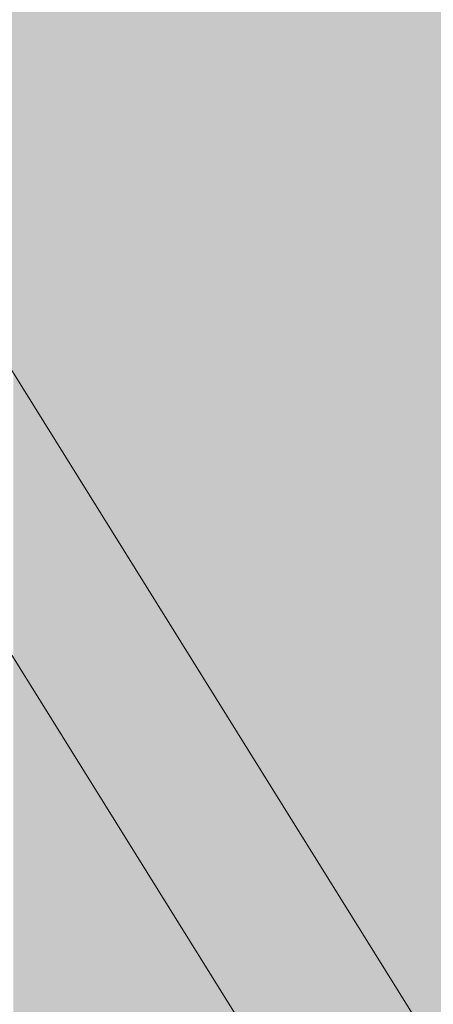
# Model space of a CAD drawing. Units: millimetres. Extents: x 11032 to 26788, y 3406 to 24505.
# Tile 51 of 78: x 15786 to 15924, y 16039 to 16366. Entities that reach past the tile are written whole.
import ezdxf

# ---------------------------------------------------------------- set-up
doc = ezdxf.new("R2010")
doc.units = ezdxf.units.MM
doc.header["$MEASUREMENT"] = 0
for name, color, linetype, lineweight in [('A-ANNO-DIMS', 2, 'Continuous', 18), ('A-GLAZ', 250, 'Continuous', 20), ('A-ROOF', 7, 'Continuous', 30), ('A-WALL', 7, 'Continuous', 35), ('E-LITE', 7, 'Continuous', 18), ('E-LITE-PATT', 7, 'Continuous', 13)]:
    doc.layers.add(name, color=color, linetype=linetype, lineweight=lineweight)
doc.layers.add('A-GLAZ-FRAM-PATT', color=250, linetype='Continuous', lineweight=13, true_color=0x262627)
doc.layers.add('A-ROOF-PATT', color=9, linetype='Continuous', lineweight=13, true_color=0xc7c8ca)
doc.styles.get("Standard").update_dxf_attribs({"font": 'arial.ttf'})
doc.dimstyles.get("Standard").update_dxf_attribs({"dimtxt": 150, "dimasz": 100, "dimexe": 10, "dimexo": 5, "dimgap": 5, "dimtad": 0, "dimtih": 1, "dimtoh": 1, "dimdec": 0, "dimzin": 0, "dimdsep": 46, "dimtxsty": 'Standard', "dimcen": 0.09, "dimadec": 0, "dimazin": 0, "dimtfac": 1, "dimtdec": 0, "dimtofl": 0, "dimtmove": 0, "dimatfit": 3, "dimfxl": 1, "dimtolj": 1, "dimtzin": 0, "dimarcsym": 0})

# ---------------------------------------------------------------- blocks, each defined once
blk = doc.blocks.new('*D36')
at = {"layer": 'A-ANNO-DIMS', "color": 0, "lineweight": -2, "transparency": 16777216}
for p, q in [((12301.26, 17115.89), (12301.26, 24416.86)), ((25397.4, 4466.4), (25397.4, 24416.86)), ((12401.26, 24406.86), (18569.2, 24406.86)), ((25297.4, 24406.86), (19129.47, 24406.86))]:
    blk.add_line(p, q, dxfattribs=at)
at = {"layer": 'A-ANNO-DIMS', "color": 0, "transparency": 16777216}
for points in [[(12401.26, 24423.52), (12401.26, 24390.19), (12301.26, 24406.86)], [(25297.4, 24423.52), (25297.4, 24390.19), (25397.4, 24406.86)]]:
    blk.add_solid(points, dxfattribs=at)
at = {"layer": 'Defpoints', "color": 0, "transparency": 16777216}
for p in [(25397.4, 24406.86), (12301.26, 17110.89), (25397.4, 4461.4)]:
    blk.add_point(p, dxfattribs=at)
at = {"layer": 'A-ANNO-DIMS', "color": 0, "transparency": 16777216, "insert": (18849.33, 24406.86), "char_height": 150, "attachment_point": 5}
blk.add_mtext('\\A1;13096', dxfattribs=at)
blk = doc.blocks.new('*D37')
at = {"layer": 'A-ANNO-DIMS', "color": 0, "lineweight": -2, "transparency": 16777216}
for p, q in [((18087.74, 23450.36), (11334.76, 23450.36)), ((11344.76, 23350.36), (11344.76, 14037.46)), ((11344.76, 4561.4), (11344.76, 13874.29)), ((12927.66, 4461.4), (11334.76, 4461.4))]:
    blk.add_line(p, q, dxfattribs=at)
at = {"layer": 'A-ANNO-DIMS', "color": 0, "transparency": 16777216}
for points in [[(11328.1, 23350.36), (11361.43, 23350.36), (11344.76, 23450.36)], [(11328.1, 4561.4), (11361.43, 4561.4), (11344.76, 4461.4)]]:
    blk.add_solid(points, dxfattribs=at)
at = {"layer": 'Defpoints', "color": 0, "transparency": 16777216}
for p in [(11344.76, 23450.36), (18092.74, 23450.36), (12932.66, 4461.4)]:
    blk.add_point(p, dxfattribs=at)
at = {"layer": 'A-ANNO-DIMS', "color": 0, "transparency": 16777216, "insert": (11344.76, 13955.88), "char_height": 150, "attachment_point": 5}
blk.add_mtext('\\A1;18989', dxfattribs=at)
blk = doc.blocks.new('*D45')
at = {"layer": 'A-ANNO-DIMS', "color": 0, "lineweight": -2, "transparency": 16777216}
for p, q in [((13792.37, 18518.92), (26363.9, 18518.92)), ((26353.9, 18418.92), (26353.9, 17450.32)), ((26353.9, 16318.44), (26353.9, 17287.05)), ((22902.4, 16218.44), (26363.9, 16218.44))]:
    blk.add_line(p, q, dxfattribs=at)
at = {"layer": 'A-ANNO-DIMS', "color": 0, "transparency": 16777216}
for points in [[(26337.24, 18418.92), (26370.57, 18418.92), (26353.9, 18518.92)], [(26337.24, 16318.44), (26370.57, 16318.44), (26353.9, 16218.44)]]:
    blk.add_solid(points, dxfattribs=at)
at = {"layer": 'Defpoints', "color": 0, "transparency": 16777216}
for p in [(13787.37, 18518.92), (26353.9, 18518.92), (22897.4, 16218.44)]:
    blk.add_point(p, dxfattribs=at)
at = {"layer": 'A-ANNO-DIMS', "color": 0, "transparency": 16777216, "insert": (26353.9, 17368.68), "char_height": 150, "attachment_point": 5}
blk.add_mtext('\\A1;2300.5', dxfattribs=at)
blk = doc.blocks.new('*D57')
at = {"layer": 'A-ANNO-DIMS', "color": 0, "lineweight": -2, "transparency": 16777216}
for p, q in [((14994.7, 7266.4), (14994.7, 24416.86)), ((20894.7, 7266.4), (20894.7, 24416.86)), ((15094.7, 24406.86), (17715.98, 24406.86)), ((20794.7, 24406.86), (18173.42, 24406.86))]:
    blk.add_line(p, q, dxfattribs=at)
at = {"layer": 'A-ANNO-DIMS', "color": 0, "transparency": 16777216}
for points in [[(15094.7, 24423.52), (15094.7, 24390.19), (14994.7, 24406.86)], [(20794.7, 24423.52), (20794.7, 24390.19), (20894.7, 24406.86)]]:
    blk.add_solid(points, dxfattribs=at)
at = {"layer": 'Defpoints', "color": 0, "transparency": 16777216}
for p in [(20894.7, 24406.86), (14994.7, 7261.4), (20894.7, 7261.4)]:
    blk.add_point(p, dxfattribs=at)
at = {"layer": 'A-ANNO-DIMS', "color": 0, "transparency": 16777216, "insert": (17944.7, 24406.86), "char_height": 150, "attachment_point": 5}
blk.add_mtext('\\A1;5900', dxfattribs=at)
blk = doc.blocks.new('*D60')
at = {"layer": 'A-ANNO-DIMS', "color": 0, "lineweight": -2, "transparency": 16777216}
for p, q in [((14994.7, 7266.4), (14994.7, 24416.86)), ((16344.7, 7266.4), (16344.7, 24416.86)), ((15094.7, 24406.86), (15448.04, 24406.86)), ((16244.7, 24406.86), (15891.36, 24406.86))]:
    blk.add_line(p, q, dxfattribs=at)
at = {"layer": 'A-ANNO-DIMS', "color": 0, "transparency": 16777216}
for points in [[(15094.7, 24423.52), (15094.7, 24390.19), (14994.7, 24406.86)], [(16244.7, 24423.52), (16244.7, 24390.19), (16344.7, 24406.86)]]:
    blk.add_solid(points, dxfattribs=at)
at = {"layer": 'Defpoints', "color": 0, "transparency": 16777216}
for p in [(16344.7, 24406.86), (14994.7, 7261.4), (16344.7, 7261.4)]:
    blk.add_point(p, dxfattribs=at)
at = {"layer": 'A-ANNO-DIMS', "color": 0, "transparency": 16777216, "insert": (15669.7, 24406.86), "char_height": 150, "attachment_point": 5}
blk.add_mtext('\\A1;1350', dxfattribs=at)

msp = doc.modelspace()

# ---------------------------------------------------------------- hatches: boundary and pattern name
at = {"layer": 'A-GLAZ-FRAM-PATT'}
h = msp.add_hatch(color=256, dxfattribs=at)
edge = h.paths.add_edge_path()
edge.add_line((15784.393, 16248.213), (15784.393, 16153.61))
edge.add_line((15784.393, 16153.61), (16560.042, 14907.752))
edge.add_spline(control_points=[(16560.042, 14907.752), (16569.192, 14907.664), (16578.343, 14907.575), (16587.493, 14907.486), (16598.103, 14907.383), (16608.713, 14907.281), (16619.296, 14907.181)], knot_values=[1012.2878735, 1012.2878735, 1012.2878735, 1012.2878735, 1027.155312, 1027.155312, 1027.155312, 1044.3939449, 1044.3939449, 1044.3939449, 1044.3939449], degree=3, periodic=0)
edge.add_line((16619.296, 14907.181), (15784.393, 16248.213))
at = {"layer": 'A-ROOF-PATT'}
h = msp.add_hatch(color=256, dxfattribs=at)
edge = h.paths.add_edge_path()
edge.add_spline(control_points=[(17532.827, 17324.837), (17391.335, 17349.016), (16840.872, 17494.912), (16080.055, 18069.544), (14738.803, 18299.641), (13382.429, 18838.336), (12580.532, 17870.207), (12430.422, 17563.822)], knot_values=[2977.6027945, 2977.6027945, 2977.6027945, 2977.6027945, 3438.1840601, 4811.6463022, 5622.8675483, 7588.0288188, 8560.6685791, 8560.6685791, 8560.6685791, 8560.6685791], degree=3, periodic=0)
edge.add_spline(control_points=[(12430.422, 17563.822), (12437.904, 17573.36), (12445.386, 17582.899), (12452.869, 17592.437), (12452.869, 17592.438), (12452.869, 17592.438), (12452.869, 17592.438)], knot_values=[1408.564138, 1408.564138, 1408.564138, 1408.564138, 1444.85989, 1444.85989, 1444.85989, 1444.8601183, 1444.8601183, 1444.8601183, 1444.8601183], degree=3, periodic=0)
edge.add_spline(control_points=[(12452.869, 17592.438), (12555.432, 17723.185), (12736.557, 17929.686), (13044.86, 18114.643), (13219.943, 18189.644), (13299.92, 18220.646)], knot_values=[339.318246, 339.318246, 339.318246, 339.318246, 836.8349967, 1151.2512933, 1408.564138, 1408.564138, 1408.564138, 1408.564138], degree=3, periodic=0)
edge.add_spline(control_points=[(13299.92, 18220.646), (13299.998, 18220.689), (13300.077, 18220.732), (13319.738, 18231.488), (13339.24, 18241.402), (13388.645, 18264.703), (13418.466, 18277.069), (13478.019, 18298.648), (13507.751, 18307.861), (13544.561, 18317.488), (13551.584, 18319.245), (13558.612, 18320.924)], knot_values=[3783.8950972, 3783.8950972, 3783.8950972, 3783.8950972, 3784.1737101, 3784.1737101, 3853.4666747, 3853.4666747, 3960.2401917, 3960.2401917, 4067.0137087, 4067.0137087, 4092.1744649, 4092.1744649, 4092.1744649, 4092.1744649], degree=3, periodic=0)
edge.add_spline(control_points=[(13558.612, 18320.924), (13581.407, 18326.373), (13604.25, 18331.007), (13657.184, 18339.957), (13687.338, 18343.732), (13748.098, 18348.892), (13778.704, 18350.276), (13840.46, 18350.833), (13871.609, 18350.005), (13934.496, 18346.313), (13966.232, 18343.449), (14030.297, 18335.871), (14062.625, 18331.158), (14127.853, 18320.088), (14160.753, 18313.73), (14241.357, 18296.556), (14289.343, 18284.997), (14386.31, 18259.688), (14435.291, 18245.941), (14534.161, 18217.034), (14584.049, 18201.875), (14684.682, 18170.964), (14735.427, 18155.212), (14837.763, 18123.971), (14889.354, 18108.482), (14954.971, 18089.677), (14968.586, 18085.823), (14992.391, 18079.184), (15002.566, 18076.376), (15021.739, 18071.153), (15030.731, 18068.729), (15047.707, 18064.21), (15055.694, 18062.106), (15079.815, 18055.825), (15095.905, 18051.728), (15143.966, 18039.717), (15175.729, 18032.084), (15254.84, 18013.501), (15301.798, 18002.866), (15394.186, 17981.845), (15439.615, 17971.459), (15528.833, 17950.135), (15572.62, 17939.197), (15658.477, 17916.021), (15700.546, 17903.785), (15753.633, 17886.734), (15765.446, 17882.835), (15786.574, 17875.653), (15795.915, 17872.404), (15810.108, 17867.349), (15814.99, 17865.588), (15824.736, 17862.029), (15829.611, 17860.226), (15844.241, 17854.75), (15854.002, 17851.008), (15883.312, 17839.521), (15902.885, 17831.512), (15966.355, 17804.548), (16010.39, 17784.302), (16098.838, 17741.267), (16143.25, 17718.478), (16232.497, 17671.098), (16277.332, 17646.507), (16367.515, 17596.295), (16412.862, 17570.676), (16504.202, 17519.209), (16550.194, 17493.362), (16643.009, 17442.263), (16689.831, 17417.011), (16756.517, 17382.472), (16775.937, 17372.58), (16795.455, 17362.84)], knot_values=[4092.1744649, 4092.1744649, 4092.1744649, 4092.1744649, 4173.7872258, 4173.7872258, 4280.5607428, 4280.5607428, 4387.3342598, 4387.3342598, 4494.1077768, 4494.1077768, 4600.8812939, 4600.8812939, 4707.6548109, 4707.6548109, 4814.4283279, 4814.4283279, 4967.1262405, 4967.1262405, 5119.8241531, 5119.8241531, 5272.5220657, 5272.5220657, 5425.2199783, 5425.2199783, 5577.9178908, 5577.9178908, 5617.7853319, 5617.7853319, 5647.4648479, 5647.4648479, 5673.611025, 5673.611025, 5696.747607, 5696.747607, 5743.6818903, 5743.6818903, 5837.5504571, 5837.5504571, 5979.7261046, 5979.7261046, 6121.9017521, 6121.9017521, 6264.0773996, 6264.0773996, 6406.2530471, 6406.2530471, 6447.2585849, 6447.2585849, 6480.0420882, 6480.0420882, 6497.3077062, 6497.3077062, 6514.5733242, 6514.5733242, 6549.1045602, 6549.1045602, 6618.1670322, 6618.1670322, 6772.6610171, 6772.6610171, 6927.155002, 6927.155002, 7081.6489869, 7081.6489869, 7236.1429718, 7236.1429718, 7390.6369567, 7390.6369567, 7545.1309416, 7545.1309416, 7608.1992868, 7608.1992868, 7608.1992868, 7608.1992868], degree=3, periodic=0)
edge.add_spline(control_points=[(16795.455, 17362.84), (16814.335, 17349.456), (16832.897, 17336.263), (16873.225, 17307.197), (16894.778, 17291.386), (16936.221, 17259.941), (16956.11, 17244.308), (16993.863, 17213.094), (17011.726, 17197.514), (17041.993, 17169.265), (17054.791, 17156.601), (17078.762, 17131.225), (17089.933, 17118.516), (17110.618, 17092.991), (17120.131, 17080.178), (17130.17, 17065.264), (17131.487, 17063.277), (17133.77, 17059.776), (17134.746, 17058.261), (17136.69, 17055.205), (17137.657, 17053.668), (17140.539, 17049.025), (17142.438, 17045.89), (17148.068, 17036.367), (17151.732, 17029.859), (17163.03, 17008.788), (17170.335, 16993.646), (17184.087, 16961.978), (17190.534, 16945.453), (17202.562, 16911.165), (17208.142, 16893.402), (17218.448, 16856.821), (17223.173, 16838.003), (17231.801, 16799.51), (17235.705, 16779.837), (17241.533, 16746.739), (17243.676, 16733.5), (17247.718, 16706.37), (17249.608, 16692.472), (17252.066, 16672.69), (17252.761, 16666.875), (17254.1, 16655.226), (17254.744, 16649.4), (17256.596, 16631.917), (17257.727, 16620.254), (17260.823, 16585.238), (17262.489, 16561.858), (17266.551, 16488.654), (17267.658, 16438.661), (17267.349, 16375.228), (17267.193, 16362.07), (17266.95, 16348.891)], knot_values=[15.1130472, 15.1130472, 15.1130472, 15.1130472, 82.6995146, 82.6995146, 165.3990291, 165.3990291, 248.0985437, 248.0985437, 330.7980583, 330.7980583, 397.9419458, 397.9419458, 465.0858333, 465.0858333, 532.2297209, 532.2297209, 542.533741, 542.533741, 550.3568158, 550.3568158, 558.1798906, 558.1798906, 573.8260402, 573.8260402, 605.1183395, 605.1183395, 672.7640614, 672.7640614, 740.4097834, 740.4097834, 808.0555054, 808.0555054, 875.7012273, 875.7012273, 943.3469493, 943.3469493, 987.6613492, 987.6613492, 1033.4121612, 1033.4121612, 1052.3850876, 1052.3850876, 1071.358014, 1071.358014, 1109.3038668, 1109.3038668, 1185.1955724, 1185.1955724, 1346.4419026, 1346.4419026, 1388.5586631, 1388.5586631, 1388.5586631, 1388.5586631], degree=3, periodic=0)
edge.add_spline(control_points=[(17266.95, 16348.891), (17266.95, 16348.891), (17266.95, 16348.891), (17266.95, 16348.891), (17253.182, 15602.417), (17239.414, 14855.943), (17225.646, 14109.469)], knot_values=[1388.5586631, 1388.5586631, 1388.5586631, 1388.5586631, 1388.5589654, 1388.5589654, 1388.5589654, 3774.0767661, 3774.0767661, 3774.0767661, 3774.0767661], degree=3, periodic=0)
edge.add_spline(control_points=[(17225.646, 14109.469), (17226.198, 14109.827), (17226.748, 14110.185), (17242.065, 14120.191), (17255.956, 14130.116), (17274.422, 14144.286), (17279.609, 14148.386), (17284.686, 14152.511)], knot_values=[1926.3423968, 1926.3423968, 1926.3423968, 1926.3423968, 1927.316729, 1927.316729, 1953.5121761, 1953.5121761, 1964.0732348, 1964.0732348, 1964.0732348, 1964.0732348], degree=3, periodic=0)
edge.add_spline(control_points=[(17284.686, 14152.511), (17315.791, 14194.761), (17384.413, 14446.273), (17407.128, 14793.401), (17407.093, 15295.84), (17423.274, 15626.362), (17415.601, 15782.507)], knot_values=[0, 0, 0, 0, 163.2554674, 619.2296767, 1171.8624483, 1621.6355562, 1621.6355562, 1621.6355562, 1621.6355562], degree=3, periodic=0)
edge.add_spline(control_points=[(17415.601, 15782.507), (17438.21, 16077.57), (17410.495, 16533.484), (17390.893, 17030.649), (17301.082, 17169.349)], knot_values=[543.9784753, 543.9784753, 543.9784753, 543.9784753, 1452.9852767, 1960.0114926, 1960.0114926, 1960.0114926, 1960.0114926], degree=3, periodic=0)
edge.add_spline(control_points=[(17301.082, 17169.349), (17346.58, 17157.64), (17392.235, 17147.336), (17467.161, 17132.609), (17496.336, 17127.412), (17525.58, 17122.709)], knot_values=[8131.593939, 8131.593939, 8131.593939, 8131.593939, 8269.7349273, 8269.7349273, 8357.5016646, 8357.5016646, 8357.5016646, 8357.5016646], degree=3, periodic=0)
edge.add_line((17525.58, 17122.709), (17532.827, 17324.837))
edge = h.paths.add_edge_path(flags=17)
edge.add_spline(control_points=[(13340.537, 14602.706), (13316.172, 14726.456), (13323.666, 14932.342), (13637.836, 15081.117), (13863.248, 15171.051), (14002.1, 15224.503), (14058.539, 15244.876)], knot_values=[680.8931862, 680.8931862, 680.8931862, 680.8931862, 1033.4728289, 1337.4008326, 1604.7214264, 1784.2944722, 1784.2944722, 1784.2944722, 1784.2944722], degree=3, periodic=0)
edge.add_spline(control_points=[(14058.539, 15244.876), (14058.289, 15275.236), (14057.634, 15305.434), (14055.312, 15376.527), (14053.359, 15417.248), (14048.642, 15497.048), (14045.89, 15536.143), (14042.888, 15574.619)], knot_values=[6573.1065419, 6573.1065419, 6573.1065419, 6573.1065419, 6636.7330012, 6636.7330012, 6723.8890547, 6723.8890547, 6809.6328771, 6809.6328771, 6809.6328771, 6809.6328771], degree=3, periodic=0)
edge.add_spline(control_points=[(14042.888, 15574.619), (13546.54, 15403.221), (13074.735, 15143.241), (13277.36, 14695.339), (13340.537, 14602.706)], knot_values=[503.7925783, 503.7925783, 503.7925783, 503.7925783, 1728.1787606, 2051.34844, 2051.34844, 2051.34844, 2051.34844], degree=3, periodic=0)
h = msp.add_hatch(color=256, dxfattribs=at)
h.set_gradient(color1=(254, 234, 185), color2=(254, 204, 102), name='HEMISPHERICAL')
edge = h.paths.add_edge_path()
edge.add_line((15084.393, 17001.32), (15284.393, 17051.32))
edge.add_line((15284.393, 17051.32), (15470.537, 16752.334))
edge.add_spline(control_points=[(15470.537, 16752.334), (15683.311, 16831.508), (16106.827, 16912.335), (16625.609, 16876.997), (17083.498, 16357.78), (17257.801, 16180.113)], knot_values=[0, 0, 0, 0, 655.2936334, 1252.0157838, 1989.6162859, 1989.6162859, 1989.6162859, 1989.6162859], degree=3, periodic=0)
edge.add_spline(control_points=[(17257.801, 16180.113), (17260.851, 16236.372), (17263.9, 16292.632), (17266.95, 16348.891)], knot_values=[1132.9967717, 1132.9967717, 1132.9967717, 1132.9967717, 1198.0464225, 1198.0464225, 1198.0464225, 1198.0464225], degree=3, periodic=0)
edge.add_spline(control_points=[(17266.95, 16348.891), (17267.193, 16362.07), (17267.349, 16375.228), (17267.658, 16438.661), (17266.551, 16488.654), (17262.489, 16561.858), (17260.823, 16585.238), (17257.727, 16620.254), (17256.596, 16631.917), (17254.744, 16649.4), (17254.1, 16655.226), (17252.761, 16666.875), (17252.066, 16672.69), (17249.608, 16692.472), (17247.718, 16706.37), (17243.676, 16733.5), (17241.533, 16746.739), (17235.705, 16779.837), (17231.801, 16799.51), (17223.173, 16838.003), (17218.448, 16856.821), (17208.142, 16893.402), (17202.562, 16911.165), (17190.534, 16945.453), (17184.087, 16961.978), (17170.335, 16993.646), (17163.03, 17008.788), (17151.732, 17029.859), (17148.068, 17036.367), (17142.438, 17045.89), (17140.539, 17049.025), (17137.657, 17053.668), (17136.69, 17055.205), (17134.746, 17058.261), (17133.77, 17059.776), (17131.487, 17063.277), (17130.17, 17065.264), (17120.131, 17080.178), (17110.618, 17092.991), (17089.933, 17118.516), (17078.762, 17131.225), (17054.791, 17156.601), (17041.993, 17169.265), (17011.726, 17197.514), (16993.863, 17213.094), (16956.11, 17244.308), (16936.221, 17259.941), (16894.778, 17291.386), (16873.225, 17307.197), (16832.897, 17336.263), (16814.335, 17349.456), (16795.455, 17362.84)], knot_values=[15.1130472, 15.1130472, 15.1130472, 15.1130472, 57.2298077, 57.2298077, 218.4761379, 218.4761379, 294.3678435, 294.3678435, 332.3136963, 332.3136963, 351.2866227, 351.2866227, 370.2595491, 370.2595491, 416.0103612, 416.0103612, 460.324761, 460.324761, 527.970483, 527.970483, 595.616205, 595.616205, 663.2619269, 663.2619269, 730.9076489, 730.9076489, 798.5533709, 798.5533709, 829.8456701, 829.8456701, 845.4918197, 845.4918197, 853.3148945, 853.3148945, 861.1379693, 861.1379693, 871.4419895, 871.4419895, 938.585877, 938.585877, 1005.7297645, 1005.7297645, 1072.8736521, 1072.8736521, 1155.5731666, 1155.5731666, 1238.2726812, 1238.2726812, 1320.9721958, 1320.9721958, 1388.5586631, 1388.5586631, 1388.5586631, 1388.5586631], degree=3, periodic=0)
edge.add_spline(control_points=[(16795.455, 17362.84), (16775.937, 17372.58), (16756.517, 17382.472), (16689.831, 17417.011), (16643.009, 17442.263), (16550.194, 17493.362), (16504.202, 17519.209), (16412.862, 17570.676), (16367.515, 17596.295), (16277.332, 17646.507), (16232.497, 17671.098), (16143.25, 17718.478), (16098.838, 17741.267), (16010.39, 17784.302), (15966.355, 17804.548), (15902.885, 17831.512), (15883.312, 17839.521), (15854.002, 17851.008), (15844.241, 17854.75), (15829.611, 17860.226), (15824.736, 17862.029), (15814.99, 17865.588), (15810.108, 17867.349), (15795.915, 17872.404), (15786.574, 17875.653), (15765.446, 17882.835), (15753.633, 17886.734), (15700.546, 17903.785), (15658.477, 17916.021), (15572.62, 17939.197), (15528.833, 17950.135), (15439.615, 17971.459), (15394.186, 17981.845), (15301.798, 18002.866), (15254.84, 18013.501), (15175.729, 18032.084), (15143.966, 18039.717), (15095.905, 18051.728), (15079.815, 18055.825), (15055.694, 18062.106), (15047.707, 18064.21), (15030.731, 18068.729), (15021.739, 18071.153), (15002.566, 18076.376), (14992.391, 18079.184), (14968.586, 18085.823), (14954.971, 18089.677), (14889.354, 18108.482), (14837.763, 18123.971), (14735.427, 18155.212), (14684.682, 18170.964), (14584.049, 18201.875), (14534.161, 18217.034), (14435.291, 18245.941), (14386.31, 18259.688), (14289.343, 18284.997), (14241.357, 18296.556), (14160.753, 18313.73), (14127.853, 18320.088), (14062.625, 18331.158), (14030.297, 18335.871), (13966.232, 18343.449), (13934.496, 18346.313), (13871.609, 18350.005), (13840.46, 18350.833), (13778.704, 18350.276), (13748.098, 18348.892), (13687.338, 18343.732), (13657.184, 18339.957), (13604.25, 18331.007), (13581.407, 18326.373), (13558.612, 18320.924)], knot_values=[4092.1744649, 4092.1744649, 4092.1744649, 4092.1744649, 4155.2428101, 4155.2428101, 4309.736795, 4309.736795, 4464.2307799, 4464.2307799, 4618.7247648, 4618.7247648, 4773.2187497, 4773.2187497, 4927.7127346, 4927.7127346, 5082.2067195, 5082.2067195, 5151.2691915, 5151.2691915, 5185.8004275, 5185.8004275, 5203.0660455, 5203.0660455, 5220.3316635, 5220.3316635, 5253.1151668, 5253.1151668, 5294.1207046, 5294.1207046, 5436.2963521, 5436.2963521, 5578.4719996, 5578.4719996, 5720.6476471, 5720.6476471, 5862.8232946, 5862.8232946, 5956.6918614, 5956.6918614, 6003.6261447, 6003.6261447, 6026.7627267, 6026.7627267, 6052.9089038, 6052.9089038, 6082.5884198, 6082.5884198, 6122.4558609, 6122.4558609, 6275.1537734, 6275.1537734, 6427.851686, 6427.851686, 6580.5495986, 6580.5495986, 6733.2475112, 6733.2475112, 6885.9454238, 6885.9454238, 6992.7189408, 6992.7189408, 7099.4924578, 7099.4924578, 7206.2659749, 7206.2659749, 7313.0394919, 7313.0394919, 7419.8130089, 7419.8130089, 7526.5865259, 7526.5865259, 7608.1992868, 7608.1992868, 7608.1992868, 7608.1992868], degree=3, periodic=0)
edge.add_spline(control_points=[(13558.612, 18320.924), (13472.381, 18287.498), (13386.15, 18254.072), (13299.92, 18220.646), (13299.92, 18220.646), (13299.92, 18220.646), (13299.92, 18220.646)], knot_values=[61.8832457, 61.8832457, 61.8832457, 61.8832457, 339.3179746, 339.3179746, 339.3179746, 339.318246, 339.318246, 339.318246, 339.318246], degree=3, periodic=0)
edge.add_spline(control_points=[(13299.92, 18220.646), (13219.943, 18189.644), (13044.86, 18114.643), (12736.557, 17929.686), (12555.432, 17723.185), (12452.869, 17592.438)], knot_values=[339.318246, 339.318246, 339.318246, 339.318246, 596.6310906, 911.0473872, 1408.564138, 1408.564138, 1408.564138, 1408.564138], degree=3, periodic=0)
edge.add_spline(control_points=[(12452.869, 17592.438), (12452.869, 17592.438), (12452.869, 17592.438), (12452.869, 17592.437), (12445.386, 17582.899), (12437.904, 17573.36), (12430.422, 17563.822)], knot_values=[1408.564138, 1408.564138, 1408.564138, 1408.564138, 1408.5643663, 1408.5643663, 1408.5643663, 1444.8601183, 1444.8601183, 1444.8601183, 1444.8601183], degree=3, periodic=0)
edge.add_spline(control_points=[(12430.422, 17563.822), (12373.797, 17448.248), (12157.302, 16836.764), (12751.985, 16393.69), (13424.325, 15907.903), (14042.888, 15574.619)], knot_values=[0, 0, 0, 0, 366.8993034, 1975.5941082, 2977.6027945, 2977.6027945, 2977.6027945, 2977.6027945], degree=3, periodic=0)
edge.add_spline(control_points=[(14042.888, 15574.619), (14042.839, 15575.252), (14042.789, 15575.886), (14039.681, 15615.607), (14036.366, 15654.052), (14029.551, 15729.305), (14026.05, 15766.114), (14019.175, 15837.686), (14015.8, 15872.45), (13903.823, 16338.596)], knot_values=[6310.2261504, 6310.2261504, 6310.2261504, 6310.2261504, 6311.6383814, 6311.6383814, 6398.7944349, 6398.7944349, 6485.9504884, 6485.9504884, 6573.1065419, 6573.1065419, 6573.1065419, 6573.1065419], degree=3, periodic=0)
edge.add_spline(control_points=[(13903.823, 16338.596), (14237.315, 16236.889), (14456.623, 16167.555), (14614.196, 16115.84)], knot_values=[0, 0, 0, 0, 202.9853419, 202.9853419, 202.9853419, 202.9853419], degree=3, periodic=0)
edge.add_spline(control_points=[(14614.196, 16115.84), (14663.209, 16178.992), (14799.965, 16341.237), (14969.915, 16481.426), (15084.393, 16556.825)], knot_values=[2405.0345045, 2405.0345045, 2405.0345045, 2405.0345045, 2644.8826966, 3039.2707272, 3039.2707272, 3039.2707272, 3039.2707272], degree=3, periodic=0)
edge.add_line((15084.393, 16556.825), (15084.393, 17001.32))
h.paths.add_polyline_path([(14195.599, 17606.181, -1), (14395.599, 17606.181, -1)], flags=16)
h.paths.add_polyline_path([(13310.178, 17032.97, -1), (13510.178, 17032.97, -1)], flags=16)
h = msp.add_hatch(color=256, dxfattribs=at)
h.set_gradient(color1=(254, 234, 185), color2=(254, 204, 102), name='HEMISPHERICAL')
edge = h.paths.add_edge_path()
edge.add_spline(control_points=[(16560.042, 14907.752), (16569.192, 14907.664), (16578.343, 14907.575), (16587.493, 14907.486), (16832.101, 14905.115), (17122.895, 14902.296), (16849.359, 14976.117), (16870.954, 15304.114), (17098.337, 15241.178), (17235.385, 15203.245)], knot_values=[0, 0, 0, 0, 14.8674385, 14.8674385, 14.8674385, 412.2943091, 487.3345915, 708.6416004, 1044.3939449, 1044.3939449, 1044.3939449, 1044.3939449], degree=3, periodic=0)
edge.add_line((16587.504, 14907.486), (16560.207, 14907.486))
edge.add_line((16560.207, 14907.486), (15784.393, 16153.61))
edge.add_line((15784.393, 16153.61), (15784.393, 15385.996))
edge.add_spline(control_points=[(15784.393, 15385.996), (15798.391, 15360.52), (15847.198, 15266.214), (15887.196, 15168.614), (15912.903, 15096.727)], knot_values=[1463.2850479, 1463.2850479, 1463.2850479, 1463.2850479, 1550.659771, 1779.9599361, 1779.9599361, 1779.9599361, 1779.9599361], degree=3, periodic=0)
edge.add_spline(control_points=[(15912.903, 15096.727), (15913.652, 15095.649), (15914.403, 15094.565), (15925.191, 15078.948), (15935.516, 15063.47), (15956.582, 15030.918), (15967.324, 15013.844), (15989.119, 14978.386), (16000.173, 14960.003), (16022.525, 14922.193), (16033.824, 14902.767), (16056.63, 14863.116), (16068.138, 14842.891), (16091.349, 14801.871), (16103.053, 14781.075), (16126.666, 14739.118), (16138.575, 14717.958), (16162.628, 14675.459), (16174.772, 14654.12), (16199.352, 14611.428), (16211.787, 14590.075), (16237.037, 14547.491), (16249.851, 14526.26), (16271.946, 14490.566), (16281.092, 14476.044), (16299.694, 14447.129), (16309.149, 14432.737), (16328.456, 14404.098), (16338.307, 14389.85), (16358.518, 14361.503), (16368.879, 14347.403), (16390.266, 14319.347), (16401.291, 14305.391), (16420.626, 14281.969), (16428.703, 14272.467), (16445.363, 14253.527), (16453.946, 14244.088), (16471.727, 14225.278), (16480.926, 14215.907), (16500.075, 14197.247), (16510.026, 14187.959), (16530.844, 14169.504), (16541.71, 14160.337), (16564.549, 14142.195), (16576.522, 14133.22), (16597.69, 14118.448), (16606.528, 14112.565), (16624.87, 14101.004), (16634.376, 14095.326), (16654.117, 14084.255), (16664.352, 14078.862), (16685.603, 14068.46), (16696.619, 14063.452), (16719.46, 14053.944), (16731.285, 14049.444), (16755.742, 14041.097), (16768.374, 14037.251), (16794.396, 14030.368), (16807.787, 14027.332), (16835.229, 14022.23), (16849.279, 14020.163), (16877.882, 14017.141), (16892.435, 14016.186), (16921.835, 14015.489), (16936.683, 14015.749), (16961.564, 14017.241), (16971.582, 14018.127), (16986.57, 14019.883), (16991.56, 14020.54), (16999.027, 14021.63), (17001.514, 14022.011), (17006.48, 14022.809), (17008.962, 14023.225), (17014.824, 14024.251), (17018.193, 14024.875), (17036.262, 14028.398), (17050.55, 14031.826), (17078.171, 14039.583), (17091.505, 14043.912), (17115.643, 14052.705), (17126.557, 14057.089), (17137.108, 14061.688)], knot_values=[2010.7639617, 2010.7639617, 2010.7639617, 2010.7639617, 2014.7029827, 2014.7029827, 2067.238337, 2067.238337, 2119.7736913, 2119.7736913, 2172.3090457, 2172.3090457, 2224.8444, 2224.8444, 2277.3797543, 2277.3797543, 2329.9151086, 2329.9151086, 2382.450463, 2382.450463, 2434.9858173, 2434.9858173, 2487.5211716, 2487.5211716, 2540.0565259, 2540.0565259, 2576.3179289, 2576.3179289, 2612.5793318, 2612.5793318, 2648.8407347, 2648.8407347, 2685.1021376, 2685.1021376, 2721.3635405, 2721.3635405, 2746.252015, 2746.252015, 2771.1404895, 2771.1404895, 2796.028964, 2796.028964, 2820.9174385, 2820.9174385, 2845.8059131, 2845.8059131, 2870.6943876, 2870.6943876, 2887.5132757, 2887.5132757, 2904.3321639, 2904.3321639, 2921.1510521, 2921.1510521, 2937.9699402, 2937.9699402, 2954.7888284, 2954.7888284, 2971.6077166, 2971.6077166, 2988.4266047, 2988.4266047, 3005.2454929, 3005.2454929, 3022.0643811, 3022.0643811, 3038.8832692, 3038.8832692, 3050.1975453, 3050.1975453, 3055.8546833, 3055.8546833, 3058.6832524, 3058.6832524, 3061.5118214, 3061.5118214, 3065.3934173, 3065.3934173, 3082.4668716, 3082.4668716, 3099.5403259, 3099.5403259, 3114.5433443, 3114.5433443, 3114.5433443, 3114.5433443], degree=3, periodic=0)
edge.add_spline(control_points=[(17137.108, 14061.688), (17165.253, 14274.398), (17209.97, 14653.885), (17230.2, 15035.586), (17235.385, 15203.245)], knot_values=[1968.0804557, 1968.0804557, 1968.0804557, 1968.0804557, 2611.5282875, 3114.5379264, 3114.5379264, 3114.5379264, 3114.5379264], degree=3, periodic=0)
edge = h.paths.add_edge_path()
edge.add_spline(control_points=[(16856.103, 14956.992), (16852.841, 14961.219), (16849.83, 14965.576), (16842.539, 14977.287), (16838.658, 14984.798), (16832.033, 15000.109), (16829.289, 15007.911), (16824.126, 15026.008), (16822.047, 15036.354), (16819.308, 15057.097), (16818.649, 15067.496), (16818.576, 15088.188), (16819.162, 15098.483), (16821.467, 15118.823), (16823.186, 15128.868), (16827.696, 15148.567), (16830.486, 15158.22), (16836.065, 15173.969), (16838.565, 15180.211), (16844.079, 15192.402), (16847.092, 15198.353), (16852.029, 15207.021), (16853.744, 15209.868), (16857.321, 15215.468), (16859.188, 15218.226), (16863.017, 15223.558), (16864.978, 15226.136), (16872.565, 15235.558), (16878.593, 15241.952), (16891.428, 15253.591), (16898.232, 15258.834), (16912.397, 15268.127), (16919.756, 15272.176), (16934.816, 15279.138), (16942.515, 15282.052), (16958.1, 15286.873), (16965.985, 15288.78), (16984.013, 15292.142), (16994.186, 15293.334), (17014.631, 15294.619), (17024.904, 15294.713), (17048.453, 15293.935), (17061.76, 15292.783), (17088.519, 15289.422), (17101.972, 15287.211), (17131.961, 15281.46), (17148.526, 15277.734), (17181.692, 15269.627), (17198.292, 15265.245), (17222.182, 15258.759), (17229.535, 15256.737), (17236.862, 15254.714)], knot_values=[9.6639535, 9.6639535, 9.6639535, 9.6639535, 20.0351668, 20.0351668, 36.9411752, 36.9411752, 53.8471837, 53.8471837, 75.7795687, 75.7795687, 97.7119538, 97.7119538, 119.6443388, 119.6443388, 141.5767238, 141.5767238, 163.5091089, 163.5091089, 178.3829945, 178.3829945, 193.2568801, 193.2568801, 200.6938229, 200.6938229, 208.1307657, 208.1307657, 215.4448585, 215.4448585, 235.5795923, 235.5795923, 255.7143261, 255.7143261, 275.8490598, 275.8490598, 295.9837936, 295.9837936, 316.1185274, 316.1185274, 341.7220543, 341.7220543, 367.3255812, 367.3255812, 400.1572431, 400.1572431, 432.988905, 432.988905, 473.0440165, 473.0440165, 513.099128, 513.099128, 530.9692999, 530.9692999, 530.9692999, 530.9692999], degree=3, periodic=0)
edge.add_spline(control_points=[(17236.862, 15254.714), (17240.377, 15387.456), (17242.496, 15609.536), (17239.752, 15831.567), (17250.544, 16044.717)], knot_values=[1250.9818616, 1250.9818616, 1250.9818616, 1250.9818616, 1649.1516581, 1916.613987, 1916.613987, 1916.613987, 1916.613987], degree=3, periodic=0)
edge.add_spline(control_points=[(17250.544, 16044.717), (17229.169, 16066.505), (17207.794, 16088.292), (17186.419, 16110.08), (17186.418, 16110.08), (17186.418, 16110.081), (17186.418, 16110.081)], knot_values=[-88.5185581, -88.5185581, -88.5185581, -88.5185581, -0.0012784, -0.0012784, -0.0012784, 0, 0, 0, 0], degree=3, periodic=0)
edge.add_spline(control_points=[(17186.418, 16110.081), (17169.261, 16127.569), (17151.499, 16145.947), (17114.892, 16184.084), (17096.046, 16203.842), (17057.437, 16244.305), (17037.673, 16265.01), (16997.415, 16306.918), (16976.921, 16328.12), (16927.79, 16378.347), (16898.924, 16407.388), (16840.771, 16464.327), (16811.484, 16492.225), (16758.449, 16540.764), (16734.666, 16561.798), (16687.634, 16601.588), (16664.382, 16620.344), (16624.116, 16650.909), (16606.897, 16663.324), (16583.769, 16678.999), (16577.49, 16683.149), (16567.144, 16689.805), (16563.039, 16692.397), (16550.823, 16699.959), (16542.775, 16704.739), (16526.841, 16713.814), (16518.956, 16718.108), (16495.524, 16730.301), (16480.199, 16737.514), (16449.97, 16750.334), (16435.066, 16755.942), (16405.476, 16765.764), (16390.79, 16769.979), (16361.418, 16777.195), (16346.731, 16780.197), (16317.147, 16785.133), (16302.249, 16787.067), (16272.053, 16789.992), (16256.756, 16790.981), (16225.609, 16792.125), (16209.759, 16792.279), (16177.385, 16791.865), (16160.862, 16791.296), (16136.98, 16790.07), (16129.942, 16789.661), (16118.22, 16788.91), (16113.574, 16788.594), (16103.645, 16787.886), (16098.362, 16787.489), (16087.761, 16786.652), (16082.439, 16786.212), (16066.413, 16784.825), (16055.649, 16783.812), (16023.135, 16780.505), (16001.164, 16777.942), (15934.539, 16769.141), (15889.17, 16761.791), (15797.417, 16743.949), (15751.033, 16733.457), (15645.217, 16705.796), (15585.74, 16687.58), (15526.207, 16666.217), (15525.367, 16665.915), (15524.528, 16665.613)], knot_values=[0, 0, 0, 0, 71.0501454, 71.0501454, 142.1002909, 142.1002909, 213.1504363, 213.1504363, 284.2005818, 284.2005818, 381.323193, 381.323193, 478.4458043, 478.4458043, 557.8219847, 557.8219847, 637.1981651, 637.1981651, 698.3122593, 698.3122593, 721.3971375, 721.3971375, 736.7790891, 736.7790891, 767.5429924, 767.5429924, 798.3068957, 798.3068957, 859.8347022, 859.8347022, 921.3625088, 921.3625088, 982.8903154, 982.8903154, 1044.4181219, 1044.4181219, 1105.9459285, 1105.9459285, 1167.4737351, 1167.4737351, 1229.0015416, 1229.0015416, 1290.5293482, 1290.5293482, 1315.8990035, 1315.8990035, 1332.3812792, 1332.3812792, 1350.9052657, 1350.9052657, 1369.4292522, 1369.4292522, 1406.4772252, 1406.4772252, 1480.5731712, 1480.5731712, 1628.7650633, 1628.7650633, 1776.9569554, 1776.9569554, 1966.3109251, 1966.3109251, 1969.019495, 1969.019495, 1969.019495, 1969.019495], degree=3, periodic=0)
edge.add_line((15524.528, 16665.613), (16587.978, 14957.484))
edge.add_spline(control_points=[(16587.978, 14957.484), (16605.253, 14957.316), (16622.516, 14957.149), (16665.945, 14956.759), (16691.933, 14956.554), (16742.419, 14956.302), (16766.918, 14956.255), (16813.531, 14956.412), (16835.647, 14956.617), (16856.103, 14956.992)], knot_values=[872.2181925, 872.2181925, 872.2181925, 872.2181925, 900.2857301, 900.2857301, 943.3659889, 943.3659889, 986.4462476, 986.4462476, 1029.5265064, 1029.5265064, 1029.5265064, 1029.5265064], degree=3, periodic=0)
h.paths.add_polyline_path([(16474.605, 15622.642, -1), (16624.605, 15622.642, -1)], flags=16)
h.paths.add_polyline_path([(16198.536, 16037.613, -1), (16348.536, 16037.613, -1)], flags=16)
h.paths.add_polyline_path([(16475.717, 16408.125, -1), (16625.717, 16408.125, -1)], flags=16)
at = {"layer": 'E-LITE-PATT'}
h = msp.add_hatch(color=256, dxfattribs=at)
edge = h.paths.add_edge_path()
edge.add_spline(control_points=[(15084.393, 16556.825), (14969.915, 16481.426), (14799.965, 16341.237), (14663.209, 16178.992), (14614.196, 16115.84)], knot_values=[2405.0345045, 2405.0345045, 2405.0345045, 2405.0345045, 2799.422535, 3039.2707272, 3039.2707272, 3039.2707272, 3039.2707272], degree=3, periodic=0)
edge.add_spline(control_points=[(14614.196, 16115.84), (14650.957, 16103.776), (14684.357, 16092.67), (14715.064, 16082.336)], knot_values=[202.9853419, 202.9853419, 202.9853419, 202.9853419, 250.3408615, 250.3408615, 250.3408615, 250.3408615], degree=3, periodic=0)
edge.add_spline(control_points=[(14715.064, 16082.336), (14732.32, 16103.979), (14749.873, 16125.274), (14780.086, 16160.475), (14792.544, 16174.592), (14817.876, 16202.424), (14830.748, 16216.137), (14853.903, 16239.975), (14864.109, 16250.213), (14884.415, 16270.066), (14894.503, 16279.688), (14918.667, 16302.183), (14932.865, 16314.967), (14987.375, 16362.454), (15029.339, 16395.81), (15076.718, 16430.13), (15080.55, 16432.882), (15084.393, 16435.621)], knot_values=[2472.5855096, 2472.5855096, 2472.5855096, 2472.5855096, 2558.786533, 2558.786533, 2617.7975153, 2617.7975153, 2676.8084975, 2676.8084975, 2721.9976237, 2721.9976237, 2765.3424393, 2765.3424393, 2824.4059302, 2824.4059302, 2988.2351723, 2988.2351723, 3002.5987883, 3002.5987883, 3002.5987883, 3002.5987883], degree=3, periodic=0)
edge.add_line((15084.393, 16435.621), (15084.393, 16556.825))
edge = h.paths.add_edge_path()
edge.add_spline(control_points=[(17257.801, 16180.113), (17083.498, 16357.78), (16625.609, 16876.997), (16106.827, 16912.335), (15683.311, 16831.508), (15470.537, 16752.334)], knot_values=[0, 0, 0, 0, 737.600502, 1334.3226525, 1989.6162859, 1989.6162859, 1989.6162859, 1989.6162859], degree=3, periodic=0)
edge.add_line((15470.537, 16752.334), (15524.528, 16665.613))
edge.add_spline(control_points=[(15524.528, 16665.613), (15525.367, 16665.915), (15526.207, 16666.217), (15585.74, 16687.58), (15645.217, 16705.796), (15751.033, 16733.457), (15797.417, 16743.949), (15889.17, 16761.791), (15934.539, 16769.141), (16001.164, 16777.942), (16023.135, 16780.505), (16055.649, 16783.812), (16066.413, 16784.825), (16082.439, 16786.212), (16087.761, 16786.652), (16098.362, 16787.489), (16103.645, 16787.886), (16113.574, 16788.594), (16118.22, 16788.91), (16129.942, 16789.661), (16136.98, 16790.07), (16160.862, 16791.296), (16177.385, 16791.865), (16209.759, 16792.279), (16225.609, 16792.125), (16256.756, 16790.981), (16272.053, 16789.992), (16302.249, 16787.067), (16317.147, 16785.133), (16346.731, 16780.197), (16361.418, 16777.195), (16390.79, 16769.979), (16405.476, 16765.764), (16435.066, 16755.942), (16449.97, 16750.334), (16480.199, 16737.514), (16495.524, 16730.301), (16518.956, 16718.108), (16526.841, 16713.814), (16542.775, 16704.739), (16550.823, 16699.959), (16563.039, 16692.397), (16567.144, 16689.805), (16577.49, 16683.149), (16583.769, 16678.999), (16606.897, 16663.324), (16624.116, 16650.909), (16664.382, 16620.344), (16687.634, 16601.588), (16734.666, 16561.798), (16758.449, 16540.764), (16811.484, 16492.225), (16840.771, 16464.327), (16898.924, 16407.388), (16927.79, 16378.347), (16976.921, 16328.12), (16997.415, 16306.918), (17037.673, 16265.01), (17057.437, 16244.305), (17096.046, 16203.842), (17114.892, 16184.084), (17151.499, 16145.947), (17169.261, 16127.569), (17186.418, 16110.081)], knot_values=[0, 0, 0, 0, 2.7085699, 2.7085699, 192.0625397, 192.0625397, 340.2544317, 340.2544317, 488.4463238, 488.4463238, 562.5422698, 562.5422698, 599.5902428, 599.5902428, 618.1142294, 618.1142294, 636.6382159, 636.6382159, 653.1204915, 653.1204915, 678.4901469, 678.4901469, 740.0179534, 740.0179534, 801.54576, 801.54576, 863.0735665, 863.0735665, 924.6013731, 924.6013731, 986.1291797, 986.1291797, 1047.6569862, 1047.6569862, 1109.1847928, 1109.1847928, 1170.7125993, 1170.7125993, 1201.4765026, 1201.4765026, 1232.2404059, 1232.2404059, 1247.6223576, 1247.6223576, 1270.7072358, 1270.7072358, 1331.8213299, 1331.8213299, 1411.1975103, 1411.1975103, 1490.5736908, 1490.5736908, 1587.696302, 1587.696302, 1684.8189133, 1684.8189133, 1755.8690587, 1755.8690587, 1826.9192041, 1826.9192041, 1897.9693496, 1897.9693496, 1969.019495, 1969.019495, 1969.019495, 1969.019495], degree=3, periodic=0)
edge.add_spline(control_points=[(17186.418, 16110.081), (17186.418, 16110.081), (17186.418, 16110.08), (17186.419, 16110.08), (17207.794, 16088.292), (17229.169, 16066.505), (17250.544, 16044.717)], knot_values=[-88.5185581, -88.5185581, -88.5185581, -88.5185581, -88.5172797, -88.5172797, -88.5172797, 0, 0, 0, 0], degree=3, periodic=0)
edge.add_spline(control_points=[(17250.544, 16044.717), (17251.307, 16059.803), (17252.131, 16075.51), (17253.018, 16091.882)], knot_values=[1232.05171, 1232.05171, 1232.05171, 1232.05171, 1250.9818616, 1250.9818616, 1250.9818616, 1250.9818616], degree=3, periodic=0)
edge.add_spline(control_points=[(17253.018, 16091.882), (17253.019, 16091.892), (17253.019, 16091.901), (17253.02, 16091.911), (17254.614, 16121.312), (17256.207, 16150.712), (17257.801, 16180.113)], knot_values=[1198.0464225, 1198.0464225, 1198.0464225, 1198.0464225, 1198.0576047, 1198.0576047, 1198.0576047, 1232.05171, 1232.05171, 1232.05171, 1232.05171], degree=3, periodic=0)

# ---------------------------------------------------------------- linework, layer by layer
at = {"layer": 'A-GLAZ'}
for p, q in [((15284.393, 17051.32), (16619.296, 14907.181)), ((15284.393, 16956.717), (16560.207, 14907.486))]:
    msp.add_line(p, q, dxfattribs=at)
at = {"layer": 'A-ROOF'}
msp.add_open_spline([(14042.888, 15574.619), (13424.325, 15907.903), (12751.985, 16393.69), (11963.048, 16981.495), (13249.687, 18891.056), (14738.803, 18299.641), (16080.055, 18069.544), (16966.203, 17400.251), (17654.208, 17293.942), (17944.704, 17286.735)], degree=3, knots=[0, 0, 0, 0, 1002.0086862, 2610.7034911, 3950.2425548, 5915.4038253, 6726.6250714, 8100.0873135, 8996.4318779, 8996.4318779, 8996.4318779, 8996.4318779], dxfattribs=at)
at = {"layer": 'A-WALL'}
msp.add_open_spline([(13903.823, 16338.596), (14592.588, 16128.54), (14947.845, 16001.782), (15353.854, 15853.294), (15563.925, 15701.294), (15714.647, 15512.154), (15830.664, 15306.558), (15887.196, 15168.614), (15912.903, 15096.727)], degree=3, knots=[0, 0, 0, 0, 419.2278857, 738.3518582, 1079.4682707, 1332.3824154, 1550.659771, 1779.9599361, 1779.9599361, 1779.9599361, 1779.9599361], dxfattribs=at)
at = {"layer": 'E-LITE'}
for points, knots in [([(17257.801, 16180.113), (17083.498, 16357.78), (16625.609, 16876.997), (16069.956, 16914.847), (15586.409, 16811.936), (15334.393, 16695.842)], [0, 0, 0, 0, 737.600502, 1334.3226525, 2131.0201637, 2131.0201637, 2131.0201637, 2131.0201637]), ([(17250.544, 16044.717), (17229.169, 16066.505), (17207.794, 16088.292), (17186.419, 16110.08), (17186.418, 16110.08), (17186.418, 16110.081), (17186.418, 16110.081), (17169.261, 16127.569), (17151.499, 16145.947), (17114.892, 16184.084), (17096.046, 16203.842), (17057.437, 16244.305), (17037.673, 16265.01), (16997.415, 16306.918), (16976.921, 16328.12), (16927.79, 16378.347), (16898.924, 16407.388), (16840.771, 16464.327), (16811.484, 16492.225), (16758.449, 16540.764), (16734.666, 16561.798), (16687.634, 16601.588), (16664.382, 16620.344), (16624.116, 16650.909), (16606.897, 16663.324), (16583.769, 16678.999), (16577.49, 16683.149), (16567.144, 16689.805), (16563.039, 16692.397), (16550.823, 16699.959), (16542.775, 16704.739), (16526.841, 16713.814), (16518.956, 16718.108), (16495.524, 16730.301), (16480.199, 16737.514), (16449.97, 16750.334), (16435.066, 16755.942), (16405.476, 16765.764), (16390.79, 16769.979), (16361.418, 16777.195), (16346.731, 16780.197), (16317.147, 16785.133), (16302.249, 16787.067), (16272.053, 16789.992), (16256.756, 16790.981), (16225.609, 16792.125), (16209.759, 16792.279), (16177.385, 16791.865), (16160.862, 16791.296), (16136.98, 16790.07), (16129.942, 16789.661), (16118.22, 16788.91), (16113.574, 16788.594), (16103.645, 16787.886), (16098.362, 16787.489), (16087.761, 16786.652), (16082.439, 16786.212), (16066.413, 16784.825), (16055.649, 16783.812), (16023.135, 16780.505), (16001.164, 16777.942), (15934.539, 16769.141), (15889.17, 16761.791), (15797.417, 16743.949), (15751.033, 16733.457), (15645.217, 16705.796), (15585.74, 16687.58), (15526.207, 16666.217), (15525.367, 16665.915), (15524.528, 16665.613)], [-88.5185581, -88.5185581, -88.5185581, -88.5185581, -0.0012784, -0.0012784, -0.0012784, 0, 0, 0, 71.0501454, 71.0501454, 142.1002909, 142.1002909, 213.1504363, 213.1504363, 284.2005818, 284.2005818, 381.323193, 381.323193, 478.4458043, 478.4458043, 557.8219847, 557.8219847, 637.1981651, 637.1981651, 698.3122593, 698.3122593, 721.3971375, 721.3971375, 736.7790891, 736.7790891, 767.5429924, 767.5429924, 798.3068957, 798.3068957, 859.8347022, 859.8347022, 921.3625088, 921.3625088, 982.8903154, 982.8903154, 1044.4181219, 1044.4181219, 1105.9459285, 1105.9459285, 1167.4737351, 1167.4737351, 1229.0015416, 1229.0015416, 1290.5293482, 1290.5293482, 1315.8990035, 1315.8990035, 1332.3812792, 1332.3812792, 1350.9052657, 1350.9052657, 1369.4292522, 1369.4292522, 1406.4772252, 1406.4772252, 1480.5731712, 1480.5731712, 1628.7650633, 1628.7650633, 1776.9569554, 1776.9569554, 1966.3109251, 1966.3109251, 1969.019495, 1969.019495, 1969.019495, 1969.019495])]:
    msp.add_open_spline(points, degree=3, knots=knots, dxfattribs=at)

# ---------------------------------------------------------------- dimensions: what is measured, and where the dimension line sits
at = {"layer": 'A-ANNO-DIMS'}
for base, p1, p2, picture, middle in [((25397.404, 24406.858), (12301.265, 17110.885), (25397.404, 4461.399), '*D36', (18849.334, 24406.858)), ((20894.704, 24406.858), (14994.704, 7261.399), (20894.704, 7261.399), '*D57', (17944.704, 24406.858)), ((16344.704, 24406.858), (14994.704, 7261.399), (16344.704, 7261.399), '*D60', (15669.704, 24406.858))]:
    dim = msp.add_linear_dim(base=base, p1=p1, p2=p2, dimstyle='Standard', override={"dimdec": 0, "dimlfac": 1, "dimrnd": 0, "dimzin": 0, "dimdsep": 46, "dimlunit": 2}, dxfattribs=at)
    dim.commit()
    dim.dimension.update_dxf_attribs({"geometry": picture, "text_midpoint": middle})
for base, p1, p2, override, picture, middle in [((11344.765, 23450.358), (12932.665, 4461.399), (18092.739, 23450.358), {"dimdec": 0, "dimlfac": 1, "dimrnd": 0, "dimzin": 0, "dimdsep": 46, "dimlunit": 2}, '*D37', (11344.765, 13955.879)), ((26353.904, 18518.925), (22897.404, 16218.44), (13787.367, 18518.925), {"dimdec": 1, "dimlfac": 1, "dimrnd": 0, "dimzin": 0, "dimdsep": 46, "dimlunit": 2}, '*D45', (26353.904, 17368.682))]:
    dim = msp.add_linear_dim(base=base, p1=p1, p2=p2, angle=90, dimstyle='Standard', override=override, dxfattribs=at)
    dim.commit()
    dim.dimension.update_dxf_attribs({"geometry": picture, "text_midpoint": middle})

doc.saveas('drawing.dxf')
